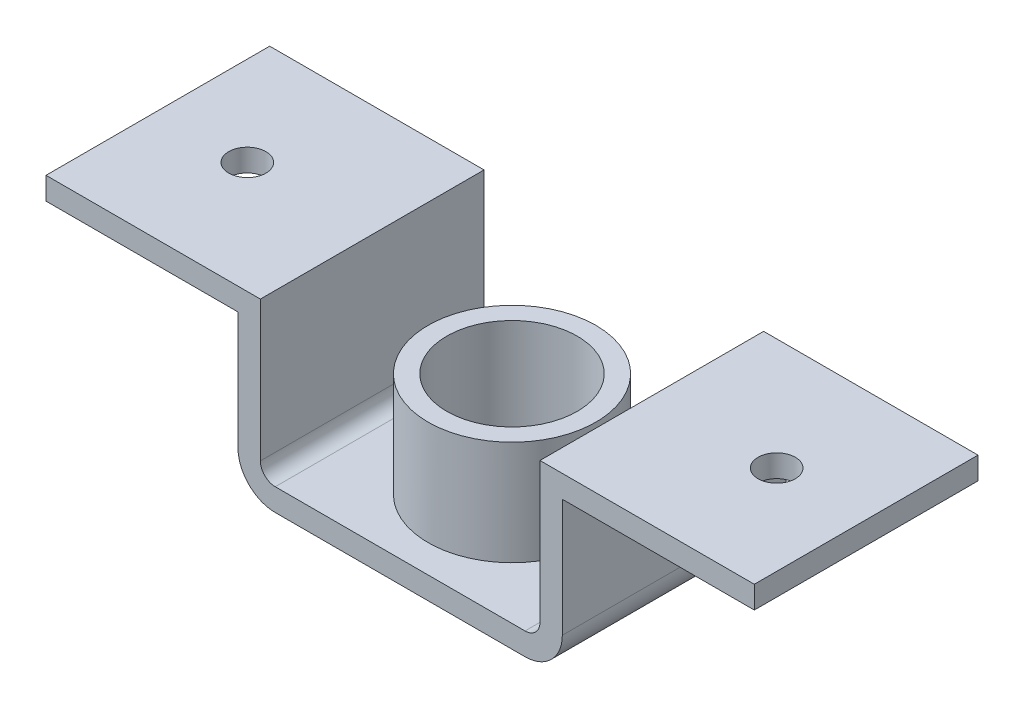
ISO-10303-21;
HEADER;
FILE_DESCRIPTION(('STEP AP214'),'2;1');
FILE_NAME('part.step','',(''),(''),'','','');
FILE_SCHEMA(('AUTOMOTIVE_DESIGN { 1 0 10303 214 1 1 1 1 }'));
ENDSEC;
DATA;
#1=APPLICATION_CONTEXT('core data for automotive mechanical design processes');
#2=APPLICATION_PROTOCOL_DEFINITION('international standard','automotive_design',2000,#1);
#3=PRODUCT_CONTEXT('',#1,'mechanical');
#4=PRODUCT('Part','Part','',(#3));
#5=PRODUCT_RELATED_PRODUCT_CATEGORY('part','',(#4));
#6=PRODUCT_DEFINITION_FORMATION('','',#4);
#7=PRODUCT_DEFINITION_CONTEXT('part definition',#1,'design');
#8=PRODUCT_DEFINITION('design','',#6,#7);
#9=PRODUCT_DEFINITION_SHAPE('','',#8);
#10=(LENGTH_UNIT() NAMED_UNIT(*) SI_UNIT(.MILLI.,.METRE.));
#11=(NAMED_UNIT(*) PLANE_ANGLE_UNIT() SI_UNIT($,.RADIAN.));
#12=(NAMED_UNIT(*) SI_UNIT($,.STERADIAN.) SOLID_ANGLE_UNIT());
#13=UNCERTAINTY_MEASURE_WITH_UNIT(LENGTH_MEASURE(1.E-05),#10,'distance_accuracy_value','');
#14=(GEOMETRIC_REPRESENTATION_CONTEXT(3) GLOBAL_UNCERTAINTY_ASSIGNED_CONTEXT((#13)) GLOBAL_UNIT_ASSIGNED_CONTEXT((#10,
#11,#12)) REPRESENTATION_CONTEXT('',''));
#15=CARTESIAN_POINT('',(0.,0.,0.));
#16=DIRECTION('',(0.,0.,1.));
#17=DIRECTION('',(1.,0.,0.));
#18=AXIS2_PLACEMENT_3D('',#15,#16,#17);
#19=CARTESIAN_POINT('',(-475.,178.,150.));
#20=DIRECTION('',(1.,0.,0.));
#21=DIRECTION('',(0.,0.,-1.));
#22=AXIS2_PLACEMENT_3D('',#19,#20,#21);
#23=PLANE('',#22);
#24=DIRECTION('',(0.,-1.,0.));
#25=VECTOR('',#24,1.);
#26=CARTESIAN_POINT('',(-475.,178.,-150.));
#27=LINE('',#26,#25);
#28=CARTESIAN_POINT('',(-475.,208.,-150.));
#29=VERTEX_POINT('',#28);
#30=CARTESIAN_POINT('',(-475.,178.,-150.));
#31=VERTEX_POINT('',#30);
#32=EDGE_CURVE('E176',#29,#31,#27,.T.);
#33=ORIENTED_EDGE('',*,*,#32,.T.);
#34=DIRECTION('',(0.,0.,-1.));
#35=VECTOR('',#34,1.);
#36=CARTESIAN_POINT('',(-475.,178.,150.));
#37=LINE('',#36,#35);
#38=CARTESIAN_POINT('',(-475.,178.,150.));
#39=VERTEX_POINT('',#38);
#40=EDGE_CURVE('E157',#39,#31,#37,.T.);
#41=ORIENTED_EDGE('',*,*,#40,.F.);
#42=DIRECTION('',(0.,-1.,0.));
#43=VECTOR('',#42,1.);
#44=CARTESIAN_POINT('',(-475.,178.,150.));
#45=LINE('',#44,#43);
#46=CARTESIAN_POINT('',(-475.,208.,150.));
#47=VERTEX_POINT('',#46);
#48=EDGE_CURVE('E165',#47,#39,#45,.T.);
#49=ORIENTED_EDGE('',*,*,#48,.F.);
#50=DIRECTION('',(0.,0.,-1.));
#51=VECTOR('',#50,1.);
#52=CARTESIAN_POINT('',(-475.,208.,150.));
#53=LINE('',#52,#51);
#54=EDGE_CURVE('E264',#47,#29,#53,.T.);
#55=ORIENTED_EDGE('',*,*,#54,.T.);
#56=EDGE_LOOP('',(#33,#41,#49,#55));
#57=FACE_BOUND('',#56,.T.);
#58=ADVANCED_FACE('F39',(#57),#23,.F.);
#59=CARTESIAN_POINT('',(-475.,178.,150.));
#60=DIRECTION('',(0.,1.,0.));
#61=DIRECTION('',(0.,0.,1.));
#62=AXIS2_PLACEMENT_3D('',#59,#60,#61);
#63=PLANE('',#62);
#64=CARTESIAN_POINT('',(-355.,178.,0.));
#65=DIRECTION('',(0.,1.,0.));
#66=DIRECTION('',(0.,0.,1.));
#67=AXIS2_PLACEMENT_3D('',#64,#65,#66);
#68=CIRCLE('',#67,25.);
#69=CARTESIAN_POINT('',(-355.,178.,25.));
#70=VERTEX_POINT('',#69);
#71=EDGE_CURVE('E327',#70,#70,#68,.T.);
#72=ORIENTED_EDGE('',*,*,#71,.T.);
#73=EDGE_LOOP('',(#72));
#74=FACE_BOUND('',#73,.T.);
#75=DIRECTION('',(1.,0.,0.));
#76=VECTOR('',#75,1.);
#77=CARTESIAN_POINT('',(-475.,178.,-150.));
#78=LINE('',#77,#76);
#79=CARTESIAN_POINT('',(-217.5,178.,-150.));
#80=VERTEX_POINT('',#79);
#81=EDGE_CURVE('E250',#31,#80,#78,.T.);
#82=ORIENTED_EDGE('',*,*,#81,.T.);
#83=DIRECTION('',(0.,0.,-1.));
#84=VECTOR('',#83,1.);
#85=CARTESIAN_POINT('',(-217.5,178.,150.));
#86=LINE('',#85,#84);
#87=CARTESIAN_POINT('',(-217.5,178.,150.));
#88=VERTEX_POINT('',#87);
#89=EDGE_CURVE('E163',#88,#80,#86,.T.);
#90=ORIENTED_EDGE('',*,*,#89,.F.);
#91=DIRECTION('',(1.,0.,0.));
#92=VECTOR('',#91,1.);
#93=CARTESIAN_POINT('',(-475.,178.,150.));
#94=LINE('',#93,#92);
#95=EDGE_CURVE('E153',#39,#88,#94,.T.);
#96=ORIENTED_EDGE('',*,*,#95,.F.);
#97=ORIENTED_EDGE('',*,*,#40,.T.);
#98=EDGE_LOOP('',(#82,#90,#96,#97));
#99=FACE_BOUND('',#98,.T.);
#100=ADVANCED_FACE('F156',(#74,#99),#63,.F.);
#101=CARTESIAN_POINT('',(-217.5,178.,150.));
#102=DIRECTION('',(1.,0.,0.));
#103=DIRECTION('',(0.,1.,0.));
#104=AXIS2_PLACEMENT_3D('',#101,#102,#103);
#105=PLANE('',#104);
#106=DIRECTION('',(0.,-1.,0.));
#107=VECTOR('',#106,1.);
#108=CARTESIAN_POINT('',(-217.5,178.,-150.));
#109=LINE('',#108,#107);
#110=CARTESIAN_POINT('',(-217.5,20.,-150.));
#111=VERTEX_POINT('',#110);
#112=EDGE_CURVE('E243',#80,#111,#109,.T.);
#113=ORIENTED_EDGE('',*,*,#112,.T.);
#114=DIRECTION('',(0.,0.,-1.));
#115=VECTOR('',#114,1.);
#116=CARTESIAN_POINT('',(-217.5,20.,150.));
#117=LINE('',#116,#115);
#118=CARTESIAN_POINT('',(-217.5,20.,150.));
#119=VERTEX_POINT('',#118);
#120=EDGE_CURVE('E11',#111,#119,#117,.F.);
#121=ORIENTED_EDGE('',*,*,#120,.T.);
#122=DIRECTION('',(0.,-1.,0.));
#123=VECTOR('',#122,1.);
#124=CARTESIAN_POINT('',(-217.5,178.,150.));
#125=LINE('',#124,#123);
#126=EDGE_CURVE('E161',#88,#119,#125,.T.);
#127=ORIENTED_EDGE('',*,*,#126,.F.);
#128=ORIENTED_EDGE('',*,*,#89,.T.);
#129=EDGE_LOOP('',(#113,#121,#127,#128));
#130=FACE_BOUND('',#129,.T.);
#131=ADVANCED_FACE('F309',(#130),#105,.F.);
#132=CARTESIAN_POINT('',(-217.5,-30.,150.));
#133=DIRECTION('',(0.,1.,0.));
#134=DIRECTION('',(0.,0.,1.));
#135=AXIS2_PLACEMENT_3D('',#132,#133,#134);
#136=PLANE('',#135);
#137=CARTESIAN_POINT('',(0.,-30.,0.));
#138=DIRECTION('',(0.,1.,0.));
#139=DIRECTION('',(0.,0.,1.));
#140=AXIS2_PLACEMENT_3D('',#137,#138,#139);
#141=CIRCLE('',#140,37.5);
#142=CARTESIAN_POINT('',(0.,-30.,37.5));
#143=VERTEX_POINT('',#142);
#144=EDGE_CURVE('E187',#143,#143,#141,.T.);
#145=ORIENTED_EDGE('',*,*,#144,.T.);
#146=EDGE_LOOP('',(#145));
#147=FACE_BOUND('',#146,.T.);
#148=DIRECTION('',(1.,0.,0.));
#149=VECTOR('',#148,1.);
#150=CARTESIAN_POINT('',(-217.5,-30.,-150.));
#151=LINE('',#150,#149);
#152=CARTESIAN_POINT('',(-167.5,-30.,-150.));
#153=VERTEX_POINT('',#152);
#154=CARTESIAN_POINT('',(167.5,-30.,-150.));
#155=VERTEX_POINT('',#154);
#156=EDGE_CURVE('E238',#153,#155,#151,.T.);
#157=ORIENTED_EDGE('',*,*,#156,.T.);
#158=DIRECTION('',(0.,0.,-1.));
#159=VECTOR('',#158,1.);
#160=CARTESIAN_POINT('',(167.5,-30.,150.));
#161=LINE('',#160,#159);
#162=CARTESIAN_POINT('',(167.5,-30.,150.));
#163=VERTEX_POINT('',#162);
#164=EDGE_CURVE('E58',#155,#163,#161,.F.);
#165=ORIENTED_EDGE('',*,*,#164,.T.);
#166=DIRECTION('',(1.,0.,0.));
#167=VECTOR('',#166,1.);
#168=CARTESIAN_POINT('',(-217.5,-30.,150.));
#169=LINE('',#168,#167);
#170=CARTESIAN_POINT('',(-167.5,-30.,150.));
#171=VERTEX_POINT('',#170);
#172=EDGE_CURVE('E223',#171,#163,#169,.T.);
#173=ORIENTED_EDGE('',*,*,#172,.F.);
#174=DIRECTION('',(0.,0.,-1.));
#175=VECTOR('',#174,1.);
#176=CARTESIAN_POINT('',(-167.5,-30.,150.));
#177=LINE('',#176,#175);
#178=EDGE_CURVE('E213',#171,#153,#177,.T.);
#179=ORIENTED_EDGE('',*,*,#178,.T.);
#180=EDGE_LOOP('',(#157,#165,#173,#179));
#181=FACE_BOUND('',#180,.T.);
#182=ADVANCED_FACE('F241',(#147,#181),#136,.F.);
#183=CARTESIAN_POINT('',(217.5,-30.,150.));
#184=DIRECTION('',(-1.,0.,0.));
#185=DIRECTION('',(0.,0.,1.));
#186=AXIS2_PLACEMENT_3D('',#183,#184,#185);
#187=PLANE('',#186);
#188=DIRECTION('',(0.,1.,0.));
#189=VECTOR('',#188,1.);
#190=CARTESIAN_POINT('',(217.5,-30.,150.));
#191=LINE('',#190,#189);
#192=CARTESIAN_POINT('',(217.5,20.,150.));
#193=VERTEX_POINT('',#192);
#194=CARTESIAN_POINT('',(217.5,178.,150.));
#195=VERTEX_POINT('',#194);
#196=EDGE_CURVE('E225',#193,#195,#191,.T.);
#197=ORIENTED_EDGE('',*,*,#196,.F.);
#198=DIRECTION('',(0.,0.,-1.));
#199=VECTOR('',#198,1.);
#200=CARTESIAN_POINT('',(217.5,20.,150.));
#201=LINE('',#200,#199);
#202=CARTESIAN_POINT('',(217.5,20.,-150.));
#203=VERTEX_POINT('',#202);
#204=EDGE_CURVE('E206',#193,#203,#201,.T.);
#205=ORIENTED_EDGE('',*,*,#204,.T.);
#206=DIRECTION('',(0.,1.,0.));
#207=VECTOR('',#206,1.);
#208=CARTESIAN_POINT('',(217.5,-30.,-150.));
#209=LINE('',#208,#207);
#210=CARTESIAN_POINT('',(217.5,178.,-150.));
#211=VERTEX_POINT('',#210);
#212=EDGE_CURVE('E239',#203,#211,#209,.T.);
#213=ORIENTED_EDGE('',*,*,#212,.T.);
#214=DIRECTION('',(0.,0.,-1.));
#215=VECTOR('',#214,1.);
#216=CARTESIAN_POINT('',(217.5,178.,150.));
#217=LINE('',#216,#215);
#218=EDGE_CURVE('E185',#195,#211,#217,.T.);
#219=ORIENTED_EDGE('',*,*,#218,.F.);
#220=EDGE_LOOP('',(#197,#205,#213,#219));
#221=FACE_BOUND('',#220,.T.);
#222=ADVANCED_FACE('F226',(#221),#187,.F.);
#223=CARTESIAN_POINT('',(217.5,178.,150.));
#224=DIRECTION('',(0.,1.,0.));
#225=DIRECTION('',(0.,0.,1.));
#226=AXIS2_PLACEMENT_3D('',#223,#224,#225);
#227=PLANE('',#226);
#228=CARTESIAN_POINT('',(355.,178.,0.));
#229=DIRECTION('',(0.,1.,0.));
#230=DIRECTION('',(0.,0.,1.));
#231=AXIS2_PLACEMENT_3D('',#228,#229,#230);
#232=CIRCLE('',#231,25.);
#233=CARTESIAN_POINT('',(355.,178.,25.));
#234=VERTEX_POINT('',#233);
#235=EDGE_CURVE('E323',#234,#234,#232,.T.);
#236=ORIENTED_EDGE('',*,*,#235,.T.);
#237=EDGE_LOOP('',(#236));
#238=FACE_BOUND('',#237,.T.);
#239=DIRECTION('',(1.,0.,0.));
#240=VECTOR('',#239,1.);
#241=CARTESIAN_POINT('',(217.5,178.,-150.));
#242=LINE('',#241,#240);
#243=CARTESIAN_POINT('',(475.,178.,-150.));
#244=VERTEX_POINT('',#243);
#245=EDGE_CURVE('E244',#211,#244,#242,.T.);
#246=ORIENTED_EDGE('',*,*,#245,.T.);
#247=DIRECTION('',(0.,0.,-1.));
#248=VECTOR('',#247,1.);
#249=CARTESIAN_POINT('',(475.,178.,150.));
#250=LINE('',#249,#248);
#251=CARTESIAN_POINT('',(475.,178.,150.));
#252=VERTEX_POINT('',#251);
#253=EDGE_CURVE('E277',#252,#244,#250,.T.);
#254=ORIENTED_EDGE('',*,*,#253,.F.);
#255=DIRECTION('',(1.,0.,0.));
#256=VECTOR('',#255,1.);
#257=CARTESIAN_POINT('',(217.5,178.,150.));
#258=LINE('',#257,#256);
#259=EDGE_CURVE('E235',#195,#252,#258,.T.);
#260=ORIENTED_EDGE('',*,*,#259,.F.);
#261=ORIENTED_EDGE('',*,*,#218,.T.);
#262=EDGE_LOOP('',(#246,#254,#260,#261));
#263=FACE_BOUND('',#262,.T.);
#264=ADVANCED_FACE('F276',(#238,#263),#227,.F.);
#265=CARTESIAN_POINT('',(475.,178.,150.));
#266=DIRECTION('',(-1.,0.,0.));
#267=DIRECTION('',(0.,0.,1.));
#268=AXIS2_PLACEMENT_3D('',#265,#266,#267);
#269=PLANE('',#268);
#270=DIRECTION('',(0.,1.,0.));
#271=VECTOR('',#270,1.);
#272=CARTESIAN_POINT('',(475.,178.,-150.));
#273=LINE('',#272,#271);
#274=CARTESIAN_POINT('',(475.,208.,-150.));
#275=VERTEX_POINT('',#274);
#276=EDGE_CURVE('E255',#244,#275,#273,.T.);
#277=ORIENTED_EDGE('',*,*,#276,.T.);
#278=DIRECTION('',(0.,0.,-1.));
#279=VECTOR('',#278,1.);
#280=CARTESIAN_POINT('',(475.,208.,150.));
#281=LINE('',#280,#279);
#282=CARTESIAN_POINT('',(475.,208.,150.));
#283=VERTEX_POINT('',#282);
#284=EDGE_CURVE('E271',#283,#275,#281,.T.);
#285=ORIENTED_EDGE('',*,*,#284,.F.);
#286=DIRECTION('',(0.,1.,0.));
#287=VECTOR('',#286,1.);
#288=CARTESIAN_POINT('',(475.,178.,150.));
#289=LINE('',#288,#287);
#290=EDGE_CURVE('E298',#252,#283,#289,.T.);
#291=ORIENTED_EDGE('',*,*,#290,.F.);
#292=ORIENTED_EDGE('',*,*,#253,.T.);
#293=EDGE_LOOP('',(#277,#285,#291,#292));
#294=FACE_BOUND('',#293,.T.);
#295=ADVANCED_FACE('F286',(#294),#269,.F.);
#296=CARTESIAN_POINT('',(187.5,208.,150.));
#297=DIRECTION('',(0.,-1.,0.));
#298=DIRECTION('',(0.,0.,-1.));
#299=AXIS2_PLACEMENT_3D('',#296,#297,#298);
#300=PLANE('',#299);
#301=CARTESIAN_POINT('',(355.,208.,0.));
#302=DIRECTION('',(0.,1.,0.));
#303=DIRECTION('',(0.,0.,-1.));
#304=AXIS2_PLACEMENT_3D('',#301,#302,#303);
#305=CIRCLE('',#304,25.);
#306=CARTESIAN_POINT('',(355.,208.,-25.));
#307=VERTEX_POINT('',#306);
#308=EDGE_CURVE('E335',#307,#307,#305,.T.);
#309=ORIENTED_EDGE('',*,*,#308,.F.);
#310=EDGE_LOOP('',(#309));
#311=FACE_BOUND('',#310,.T.);
#312=DIRECTION('',(-1.,0.,0.));
#313=VECTOR('',#312,1.);
#314=CARTESIAN_POINT('',(187.5,208.,-150.));
#315=LINE('',#314,#313);
#316=CARTESIAN_POINT('',(187.5,208.,-150.));
#317=VERTEX_POINT('',#316);
#318=EDGE_CURVE('E251',#275,#317,#315,.T.);
#319=ORIENTED_EDGE('',*,*,#318,.T.);
#320=DIRECTION('',(0.,0.,-1.));
#321=VECTOR('',#320,1.);
#322=CARTESIAN_POINT('',(187.5,208.,150.));
#323=LINE('',#322,#321);
#324=CARTESIAN_POINT('',(187.5,208.,150.));
#325=VERTEX_POINT('',#324);
#326=EDGE_CURVE('E269',#325,#317,#323,.T.);
#327=ORIENTED_EDGE('',*,*,#326,.F.);
#328=DIRECTION('',(-1.,0.,0.));
#329=VECTOR('',#328,1.);
#330=CARTESIAN_POINT('',(187.5,208.,150.));
#331=LINE('',#330,#329);
#332=EDGE_CURVE('E292',#283,#325,#331,.T.);
#333=ORIENTED_EDGE('',*,*,#332,.F.);
#334=ORIENTED_EDGE('',*,*,#284,.T.);
#335=EDGE_LOOP('',(#319,#327,#333,#334));
#336=FACE_BOUND('',#335,.T.);
#337=ADVANCED_FACE('F289',(#311,#336),#300,.F.);
#338=CARTESIAN_POINT('',(187.5,0.,150.));
#339=DIRECTION('',(1.,0.,0.));
#340=DIRECTION('',(0.,1.,0.));
#341=AXIS2_PLACEMENT_3D('',#338,#339,#340);
#342=PLANE('',#341);
#343=DIRECTION('',(0.,-1.,0.));
#344=VECTOR('',#343,1.);
#345=CARTESIAN_POINT('',(187.5,0.,-150.));
#346=LINE('',#345,#344);
#347=CARTESIAN_POINT('',(187.5,20.,-150.));
#348=VERTEX_POINT('',#347);
#349=EDGE_CURVE('E257',#317,#348,#346,.T.);
#350=ORIENTED_EDGE('',*,*,#349,.T.);
#351=DIRECTION('',(0.,0.,-1.));
#352=VECTOR('',#351,1.);
#353=CARTESIAN_POINT('',(187.5,20.,150.));
#354=LINE('',#353,#352);
#355=CARTESIAN_POINT('',(187.5,20.,150.));
#356=VERTEX_POINT('',#355);
#357=EDGE_CURVE('E193',#348,#356,#354,.F.);
#358=ORIENTED_EDGE('',*,*,#357,.T.);
#359=DIRECTION('',(0.,-1.,0.));
#360=VECTOR('',#359,1.);
#361=CARTESIAN_POINT('',(187.5,0.,150.));
#362=LINE('',#361,#360);
#363=EDGE_CURVE('E294',#325,#356,#362,.T.);
#364=ORIENTED_EDGE('',*,*,#363,.F.);
#365=ORIENTED_EDGE('',*,*,#326,.T.);
#366=EDGE_LOOP('',(#350,#358,#364,#365));
#367=FACE_BOUND('',#366,.T.);
#368=ADVANCED_FACE('F366',(#367),#342,.F.);
#369=CARTESIAN_POINT('',(-187.5,0.,150.));
#370=DIRECTION('',(0.,-1.,0.));
#371=DIRECTION('',(0.,0.,-1.));
#372=AXIS2_PLACEMENT_3D('',#369,#370,#371);
#373=PLANE('',#372);
#374=CARTESIAN_POINT('',(0.,0.,0.));
#375=DIRECTION('',(0.,-1.,0.));
#376=DIRECTION('',(0.,0.,-1.));
#377=AXIS2_PLACEMENT_3D('',#374,#375,#376);
#378=CIRCLE('',#377,112.5);
#379=CARTESIAN_POINT('',(0.,0.,-112.5));
#380=VERTEX_POINT('',#379);
#381=EDGE_CURVE('E180',#380,#380,#378,.F.);
#382=ORIENTED_EDGE('',*,*,#381,.F.);
#383=EDGE_LOOP('',(#382));
#384=FACE_BOUND('',#383,.T.);
#385=DIRECTION('',(-1.,0.,0.));
#386=VECTOR('',#385,1.);
#387=CARTESIAN_POINT('',(-187.5,0.,150.));
#388=LINE('',#387,#386);
#389=CARTESIAN_POINT('',(167.5,0.,150.));
#390=VERTEX_POINT('',#389);
#391=CARTESIAN_POINT('',(-167.5,0.,150.));
#392=VERTEX_POINT('',#391);
#393=EDGE_CURVE('E296',#390,#392,#388,.T.);
#394=ORIENTED_EDGE('',*,*,#393,.F.);
#395=DIRECTION('',(0.,0.,-1.));
#396=VECTOR('',#395,1.);
#397=CARTESIAN_POINT('',(167.5,0.,-150.));
#398=LINE('',#397,#396);
#399=CARTESIAN_POINT('',(167.5,0.,-150.));
#400=VERTEX_POINT('',#399);
#401=EDGE_CURVE('E195',#390,#400,#398,.T.);
#402=ORIENTED_EDGE('',*,*,#401,.T.);
#403=DIRECTION('',(-1.,0.,0.));
#404=VECTOR('',#403,1.);
#405=CARTESIAN_POINT('',(-187.5,0.,-150.));
#406=LINE('',#405,#404);
#407=CARTESIAN_POINT('',(-167.5,0.,-150.));
#408=VERTEX_POINT('',#407);
#409=EDGE_CURVE('E256',#400,#408,#406,.T.);
#410=ORIENTED_EDGE('',*,*,#409,.T.);
#411=DIRECTION('',(0.,0.,-1.));
#412=VECTOR('',#411,1.);
#413=CARTESIAN_POINT('',(-167.5,0.,150.));
#414=LINE('',#413,#412);
#415=EDGE_CURVE('E179',#408,#392,#414,.F.);
#416=ORIENTED_EDGE('',*,*,#415,.T.);
#417=EDGE_LOOP('',(#394,#402,#410,#416));
#418=FACE_BOUND('',#417,.T.);
#419=ADVANCED_FACE('F360',(#384,#418),#373,.F.);
#420=CARTESIAN_POINT('',(-187.5,208.,150.));
#421=DIRECTION('',(-1.,0.,0.));
#422=DIRECTION('',(0.,-1.,0.));
#423=AXIS2_PLACEMENT_3D('',#420,#421,#422);
#424=PLANE('',#423);
#425=DIRECTION('',(0.,1.,0.));
#426=VECTOR('',#425,1.);
#427=CARTESIAN_POINT('',(-187.5,208.,150.));
#428=LINE('',#427,#426);
#429=CARTESIAN_POINT('',(-187.5,20.,150.));
#430=VERTEX_POINT('',#429);
#431=CARTESIAN_POINT('',(-187.5,208.,150.));
#432=VERTEX_POINT('',#431);
#433=EDGE_CURVE('E304',#430,#432,#428,.T.);
#434=ORIENTED_EDGE('',*,*,#433,.F.);
#435=DIRECTION('',(0.,0.,-1.));
#436=VECTOR('',#435,1.);
#437=CARTESIAN_POINT('',(-187.5,20.,-150.));
#438=LINE('',#437,#436);
#439=CARTESIAN_POINT('',(-187.5,20.,-150.));
#440=VERTEX_POINT('',#439);
#441=EDGE_CURVE('E200',#430,#440,#438,.T.);
#442=ORIENTED_EDGE('',*,*,#441,.T.);
#443=DIRECTION('',(0.,1.,0.));
#444=VECTOR('',#443,1.);
#445=CARTESIAN_POINT('',(-187.5,208.,-150.));
#446=LINE('',#445,#444);
#447=CARTESIAN_POINT('',(-187.5,208.,-150.));
#448=VERTEX_POINT('',#447);
#449=EDGE_CURVE('E265',#440,#448,#446,.T.);
#450=ORIENTED_EDGE('',*,*,#449,.T.);
#451=DIRECTION('',(0.,0.,-1.));
#452=VECTOR('',#451,1.);
#453=CARTESIAN_POINT('',(-187.5,208.,150.));
#454=LINE('',#453,#452);
#455=EDGE_CURVE('E270',#432,#448,#454,.T.);
#456=ORIENTED_EDGE('',*,*,#455,.F.);
#457=EDGE_LOOP('',(#434,#442,#450,#456));
#458=FACE_BOUND('',#457,.T.);
#459=ADVANCED_FACE('F341',(#458),#424,.F.);
#460=CARTESIAN_POINT('',(-475.,208.,150.));
#461=DIRECTION('',(0.,-1.,0.));
#462=DIRECTION('',(0.,0.,-1.));
#463=AXIS2_PLACEMENT_3D('',#460,#461,#462);
#464=PLANE('',#463);
#465=CARTESIAN_POINT('',(-355.,208.,0.));
#466=DIRECTION('',(0.,1.,0.));
#467=DIRECTION('',(0.,0.,1.));
#468=AXIS2_PLACEMENT_3D('',#465,#466,#467);
#469=CIRCLE('',#468,25.);
#470=CARTESIAN_POINT('',(-355.,208.,25.));
#471=VERTEX_POINT('',#470);
#472=EDGE_CURVE('E331',#471,#471,#469,.T.);
#473=ORIENTED_EDGE('',*,*,#472,.F.);
#474=EDGE_LOOP('',(#473));
#475=FACE_BOUND('',#474,.T.);
#476=DIRECTION('',(-1.,0.,0.));
#477=VECTOR('',#476,1.);
#478=CARTESIAN_POINT('',(-475.,208.,-150.));
#479=LINE('',#478,#477);
#480=EDGE_CURVE('E173',#448,#29,#479,.T.);
#481=ORIENTED_EDGE('',*,*,#480,.T.);
#482=ORIENTED_EDGE('',*,*,#54,.F.);
#483=DIRECTION('',(-1.,0.,0.));
#484=VECTOR('',#483,1.);
#485=CARTESIAN_POINT('',(-475.,208.,150.));
#486=LINE('',#485,#484);
#487=EDGE_CURVE('E169',#432,#47,#486,.T.);
#488=ORIENTED_EDGE('',*,*,#487,.F.);
#489=ORIENTED_EDGE('',*,*,#455,.T.);
#490=EDGE_LOOP('',(#481,#482,#488,#489));
#491=FACE_BOUND('',#490,.T.);
#492=ADVANCED_FACE('F342',(#475,#491),#464,.F.);
#493=CARTESIAN_POINT('',(0.,0.,150.));
#494=DIRECTION('',(0.,0.,-1.));
#495=DIRECTION('',(-1.,0.,0.));
#496=AXIS2_PLACEMENT_3D('',#493,#494,#495);
#497=PLANE('',#496);
#498=ORIENTED_EDGE('',*,*,#172,.T.);
#499=CARTESIAN_POINT('',(167.5,20.,150.));
#500=DIRECTION('',(0.,0.,-1.));
#501=DIRECTION('',(-1.,0.,0.));
#502=AXIS2_PLACEMENT_3D('',#499,#500,#501);
#503=CIRCLE('',#502,50.);
#504=EDGE_CURVE('E50',#163,#193,#503,.F.);
#505=ORIENTED_EDGE('',*,*,#504,.T.);
#506=ORIENTED_EDGE('',*,*,#196,.T.);
#507=ORIENTED_EDGE('',*,*,#259,.T.);
#508=ORIENTED_EDGE('',*,*,#290,.T.);
#509=ORIENTED_EDGE('',*,*,#332,.T.);
#510=ORIENTED_EDGE('',*,*,#363,.T.);
#511=CARTESIAN_POINT('',(167.5,20.,150.));
#512=DIRECTION('',(0.,0.,-1.));
#513=DIRECTION('',(-1.,0.,0.));
#514=AXIS2_PLACEMENT_3D('',#511,#512,#513);
#515=CIRCLE('',#514,20.);
#516=EDGE_CURVE('E205',#356,#390,#515,.T.);
#517=ORIENTED_EDGE('',*,*,#516,.T.);
#518=ORIENTED_EDGE('',*,*,#393,.T.);
#519=CARTESIAN_POINT('',(-167.5,20.,150.));
#520=DIRECTION('',(0.,0.,-1.));
#521=DIRECTION('',(-1.,0.,0.));
#522=AXIS2_PLACEMENT_3D('',#519,#520,#521);
#523=CIRCLE('',#522,20.);
#524=EDGE_CURVE('E207',#392,#430,#523,.T.);
#525=ORIENTED_EDGE('',*,*,#524,.T.);
#526=ORIENTED_EDGE('',*,*,#433,.T.);
#527=ORIENTED_EDGE('',*,*,#487,.T.);
#528=ORIENTED_EDGE('',*,*,#48,.T.);
#529=ORIENTED_EDGE('',*,*,#95,.T.);
#530=ORIENTED_EDGE('',*,*,#126,.T.);
#531=CARTESIAN_POINT('',(-167.5,20.,150.));
#532=DIRECTION('',(0.,0.,-1.));
#533=DIRECTION('',(-1.,0.,0.));
#534=AXIS2_PLACEMENT_3D('',#531,#532,#533);
#535=CIRCLE('',#534,50.);
#536=EDGE_CURVE('E218',#119,#171,#535,.F.);
#537=ORIENTED_EDGE('',*,*,#536,.T.);
#538=EDGE_LOOP('',(#498,#505,#506,#507,#508,#509,#510,#517,#518,#525,#526,#527,#528,#529,#530,#537));
#539=FACE_BOUND('',#538,.T.);
#540=ADVANCED_FACE('F170',(#539),#497,.F.);
#541=CARTESIAN_POINT('',(0.,0.,-150.));
#542=DIRECTION('',(0.,0.,-1.));
#543=DIRECTION('',(-1.,0.,0.));
#544=AXIS2_PLACEMENT_3D('',#541,#542,#543);
#545=PLANE('',#544);
#546=ORIENTED_EDGE('',*,*,#212,.F.);
#547=CARTESIAN_POINT('',(167.5,20.,-150.));
#548=DIRECTION('',(0.,0.,-1.));
#549=DIRECTION('',(-1.,0.,0.));
#550=AXIS2_PLACEMENT_3D('',#547,#548,#549);
#551=CIRCLE('',#550,50.);
#552=EDGE_CURVE('E214',#203,#155,#551,.T.);
#553=ORIENTED_EDGE('',*,*,#552,.T.);
#554=ORIENTED_EDGE('',*,*,#156,.F.);
#555=CARTESIAN_POINT('',(-167.5,20.,-150.));
#556=DIRECTION('',(0.,0.,-1.));
#557=DIRECTION('',(-1.,0.,0.));
#558=AXIS2_PLACEMENT_3D('',#555,#556,#557);
#559=CIRCLE('',#558,50.);
#560=EDGE_CURVE('E212',#153,#111,#559,.T.);
#561=ORIENTED_EDGE('',*,*,#560,.T.);
#562=ORIENTED_EDGE('',*,*,#112,.F.);
#563=ORIENTED_EDGE('',*,*,#81,.F.);
#564=ORIENTED_EDGE('',*,*,#32,.F.);
#565=ORIENTED_EDGE('',*,*,#480,.F.);
#566=ORIENTED_EDGE('',*,*,#449,.F.);
#567=CARTESIAN_POINT('',(-167.5,20.,-150.));
#568=DIRECTION('',(0.,0.,-1.));
#569=DIRECTION('',(-1.,0.,0.));
#570=AXIS2_PLACEMENT_3D('',#567,#568,#569);
#571=CIRCLE('',#570,20.);
#572=EDGE_CURVE('E203',#440,#408,#571,.F.);
#573=ORIENTED_EDGE('',*,*,#572,.T.);
#574=ORIENTED_EDGE('',*,*,#409,.F.);
#575=CARTESIAN_POINT('',(167.5,20.,-150.));
#576=DIRECTION('',(0.,0.,-1.));
#577=DIRECTION('',(-1.,0.,0.));
#578=AXIS2_PLACEMENT_3D('',#575,#576,#577);
#579=CIRCLE('',#578,20.);
#580=EDGE_CURVE('E199',#400,#348,#579,.F.);
#581=ORIENTED_EDGE('',*,*,#580,.T.);
#582=ORIENTED_EDGE('',*,*,#349,.F.);
#583=ORIENTED_EDGE('',*,*,#318,.F.);
#584=ORIENTED_EDGE('',*,*,#276,.F.);
#585=ORIENTED_EDGE('',*,*,#245,.F.);
#586=EDGE_LOOP('',(#546,#553,#554,#561,#562,#563,#564,#565,#566,#573,#574,#581,#582,#583,#584,#585));
#587=FACE_BOUND('',#586,.T.);
#588=ADVANCED_FACE('F240',(#587),#545,.T.);
#589=CARTESIAN_POINT('',(0.,140.,0.));
#590=DIRECTION('',(0.,1.,0.));
#591=DIRECTION('',(0.,0.,1.));
#592=AXIS2_PLACEMENT_3D('',#589,#590,#591);
#593=PLANE('',#592);
#594=CARTESIAN_POINT('',(0.,140.,0.));
#595=DIRECTION('',(0.,1.,0.));
#596=DIRECTION('',(0.,0.,1.));
#597=AXIS2_PLACEMENT_3D('',#594,#595,#596);
#598=CIRCLE('',#597,112.5);
#599=CARTESIAN_POINT('',(0.,140.,112.5));
#600=VERTEX_POINT('',#599);
#601=EDGE_CURVE('E308',#600,#600,#598,.T.);
#602=ORIENTED_EDGE('',*,*,#601,.T.);
#603=EDGE_LOOP('',(#602));
#604=FACE_BOUND('',#603,.T.);
#605=CARTESIAN_POINT('',(0.,140.,0.));
#606=DIRECTION('',(0.,1.,0.));
#607=DIRECTION('',(0.,0.,1.));
#608=AXIS2_PLACEMENT_3D('',#605,#606,#607);
#609=CIRCLE('',#608,87.5);
#610=CARTESIAN_POINT('',(0.,140.,87.5));
#611=VERTEX_POINT('',#610);
#612=EDGE_CURVE('E319',#611,#611,#609,.T.);
#613=ORIENTED_EDGE('',*,*,#612,.F.);
#614=EDGE_LOOP('',(#613));
#615=FACE_BOUND('',#614,.T.);
#616=ADVANCED_FACE('F467',(#604,#615),#593,.T.);
#617=CARTESIAN_POINT('',(0.,140.,0.));
#618=DIRECTION('',(0.,-1.,0.));
#619=DIRECTION('',(0.,0.,-1.));
#620=AXIS2_PLACEMENT_3D('',#617,#618,#619);
#621=CYLINDRICAL_SURFACE('',#620,112.5);
#622=ORIENTED_EDGE('',*,*,#601,.F.);
#623=EDGE_LOOP('',(#622));
#624=FACE_BOUND('',#623,.T.);
#625=ORIENTED_EDGE('',*,*,#381,.T.);
#626=EDGE_LOOP('',(#625));
#627=FACE_BOUND('',#626,.T.);
#628=ADVANCED_FACE('F456',(#624,#627),#621,.T.);
#629=CARTESIAN_POINT('',(0.,140.,0.));
#630=DIRECTION('',(0.,-1.,0.));
#631=DIRECTION('',(0.,0.,-1.));
#632=AXIS2_PLACEMENT_3D('',#629,#630,#631);
#633=CYLINDRICAL_SURFACE('',#632,87.5);
#634=ORIENTED_EDGE('',*,*,#612,.T.);
#635=EDGE_LOOP('',(#634));
#636=FACE_BOUND('',#635,.T.);
#637=CARTESIAN_POINT('',(0.,0.,0.));
#638=DIRECTION('',(0.,1.,0.));
#639=DIRECTION('',(0.,0.,1.));
#640=AXIS2_PLACEMENT_3D('',#637,#638,#639);
#641=CIRCLE('',#640,87.5);
#642=CARTESIAN_POINT('',(0.,0.,87.5));
#643=VERTEX_POINT('',#642);
#644=EDGE_CURVE('E186',#643,#643,#641,.T.);
#645=ORIENTED_EDGE('',*,*,#644,.F.);
#646=EDGE_LOOP('',(#645));
#647=FACE_BOUND('',#646,.T.);
#648=ADVANCED_FACE('F452',(#636,#647),#633,.F.);
#649=CARTESIAN_POINT('',(0.,0.,0.));
#650=DIRECTION('',(0.,1.,0.));
#651=DIRECTION('',(0.,0.,1.));
#652=AXIS2_PLACEMENT_3D('',#649,#650,#651);
#653=CIRCLE('',#652,37.5);
#654=CARTESIAN_POINT('',(0.,0.,37.5));
#655=VERTEX_POINT('',#654);
#656=EDGE_CURVE('E188',#655,#655,#653,.T.);
#657=ORIENTED_EDGE('',*,*,#656,.F.);
#658=EDGE_LOOP('',(#657));
#659=FACE_BOUND('',#658,.T.);
#660=ORIENTED_EDGE('',*,*,#644,.T.);
#661=EDGE_LOOP('',(#660));
#662=FACE_BOUND('',#661,.T.);
#663=ADVANCED_FACE('F374',(#659,#662),#373,.F.);
#664=CARTESIAN_POINT('',(0.,-140.,0.));
#665=DIRECTION('',(0.,1.,0.));
#666=DIRECTION('',(0.,0.,1.));
#667=AXIS2_PLACEMENT_3D('',#664,#665,#666);
#668=CYLINDRICAL_SURFACE('',#667,37.5);
#669=ORIENTED_EDGE('',*,*,#656,.T.);
#670=EDGE_LOOP('',(#669));
#671=FACE_BOUND('',#670,.T.);
#672=ORIENTED_EDGE('',*,*,#144,.F.);
#673=EDGE_LOOP('',(#672));
#674=FACE_BOUND('',#673,.T.);
#675=ADVANCED_FACE('F436',(#671,#674),#668,.F.);
#676=CARTESIAN_POINT('',(-355.,68.,0.));
#677=DIRECTION('',(0.,1.,0.));
#678=DIRECTION('',(0.,0.,1.));
#679=AXIS2_PLACEMENT_3D('',#676,#677,#678);
#680=CYLINDRICAL_SURFACE('',#679,25.);
#681=ORIENTED_EDGE('',*,*,#472,.T.);
#682=EDGE_LOOP('',(#681));
#683=FACE_BOUND('',#682,.T.);
#684=ORIENTED_EDGE('',*,*,#71,.F.);
#685=EDGE_LOOP('',(#684));
#686=FACE_BOUND('',#685,.T.);
#687=ADVANCED_FACE('F336',(#683,#686),#680,.F.);
#688=CARTESIAN_POINT('',(355.,68.,0.));
#689=DIRECTION('',(0.,1.,0.));
#690=DIRECTION('',(0.,0.,1.));
#691=AXIS2_PLACEMENT_3D('',#688,#689,#690);
#692=CYLINDRICAL_SURFACE('',#691,25.);
#693=ORIENTED_EDGE('',*,*,#308,.T.);
#694=EDGE_LOOP('',(#693));
#695=FACE_BOUND('',#694,.T.);
#696=ORIENTED_EDGE('',*,*,#235,.F.);
#697=EDGE_LOOP('',(#696));
#698=FACE_BOUND('',#697,.T.);
#699=ADVANCED_FACE('F391',(#695,#698),#692,.F.);
#700=CARTESIAN_POINT('',(167.5,20.,150.));
#701=DIRECTION('',(0.,0.,1.));
#702=DIRECTION('',(1.,0.,0.));
#703=AXIS2_PLACEMENT_3D('',#700,#701,#702);
#704=CYLINDRICAL_SURFACE('',#703,20.);
#705=ORIENTED_EDGE('',*,*,#516,.F.);
#706=ORIENTED_EDGE('',*,*,#357,.F.);
#707=ORIENTED_EDGE('',*,*,#580,.F.);
#708=ORIENTED_EDGE('',*,*,#401,.F.);
#709=EDGE_LOOP('',(#705,#706,#707,#708));
#710=FACE_BOUND('',#709,.T.);
#711=ADVANCED_FACE('F364',(#710),#704,.F.);
#712=CARTESIAN_POINT('',(-167.5,20.,150.));
#713=DIRECTION('',(0.,0.,1.));
#714=DIRECTION('',(1.,0.,0.));
#715=AXIS2_PLACEMENT_3D('',#712,#713,#714);
#716=CYLINDRICAL_SURFACE('',#715,20.);
#717=ORIENTED_EDGE('',*,*,#524,.F.);
#718=ORIENTED_EDGE('',*,*,#415,.F.);
#719=ORIENTED_EDGE('',*,*,#572,.F.);
#720=ORIENTED_EDGE('',*,*,#441,.F.);
#721=EDGE_LOOP('',(#717,#718,#719,#720));
#722=FACE_BOUND('',#721,.T.);
#723=ADVANCED_FACE('F354',(#722),#716,.F.);
#724=CARTESIAN_POINT('',(167.5,20.,150.));
#725=DIRECTION('',(0.,0.,-1.));
#726=DIRECTION('',(-1.,0.,0.));
#727=AXIS2_PLACEMENT_3D('',#724,#725,#726);
#728=CYLINDRICAL_SURFACE('',#727,50.);
#729=ORIENTED_EDGE('',*,*,#504,.F.);
#730=ORIENTED_EDGE('',*,*,#164,.F.);
#731=ORIENTED_EDGE('',*,*,#552,.F.);
#732=ORIENTED_EDGE('',*,*,#204,.F.);
#733=EDGE_LOOP('',(#729,#730,#731,#732));
#734=FACE_BOUND('',#733,.T.);
#735=ADVANCED_FACE('F234',(#734),#728,.T.);
#736=CARTESIAN_POINT('',(-167.5,20.,150.));
#737=DIRECTION('',(0.,0.,-1.));
#738=DIRECTION('',(-1.,0.,0.));
#739=AXIS2_PLACEMENT_3D('',#736,#737,#738);
#740=CYLINDRICAL_SURFACE('',#739,50.);
#741=ORIENTED_EDGE('',*,*,#536,.F.);
#742=ORIENTED_EDGE('',*,*,#120,.F.);
#743=ORIENTED_EDGE('',*,*,#560,.F.);
#744=ORIENTED_EDGE('',*,*,#178,.F.);
#745=EDGE_LOOP('',(#741,#742,#743,#744));
#746=FACE_BOUND('',#745,.T.);
#747=ADVANCED_FACE('F41',(#746),#740,.T.);
#748=CLOSED_SHELL('',(#58,#100,#131,#182,#222,#264,#295,#337,#368,#419,#459,#492,#540,#588,#616,
#628,#648,#663,#675,#687,#699,#711,#723,#735,#747));
#749=MANIFOLD_SOLID_BREP('B2',#748);
#750=ADVANCED_BREP_SHAPE_REPRESENTATION('',(#18,#749),#14);
#751=SHAPE_DEFINITION_REPRESENTATION(#9,#750);
ENDSEC;
END-ISO-10303-21;
